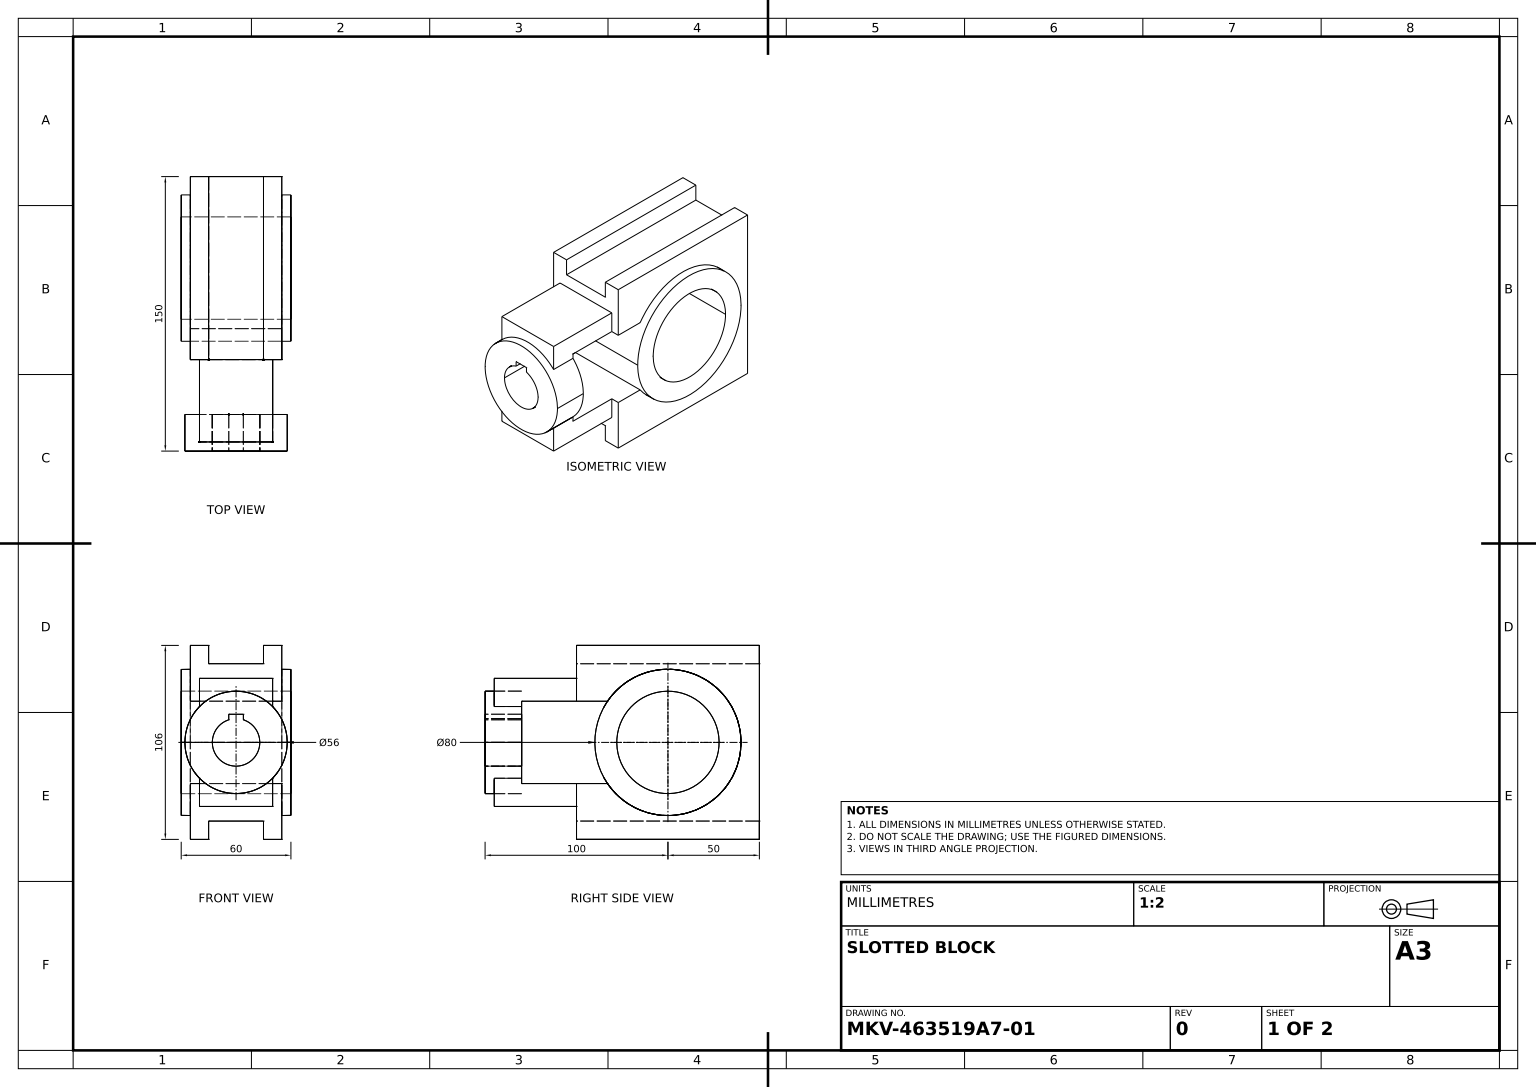
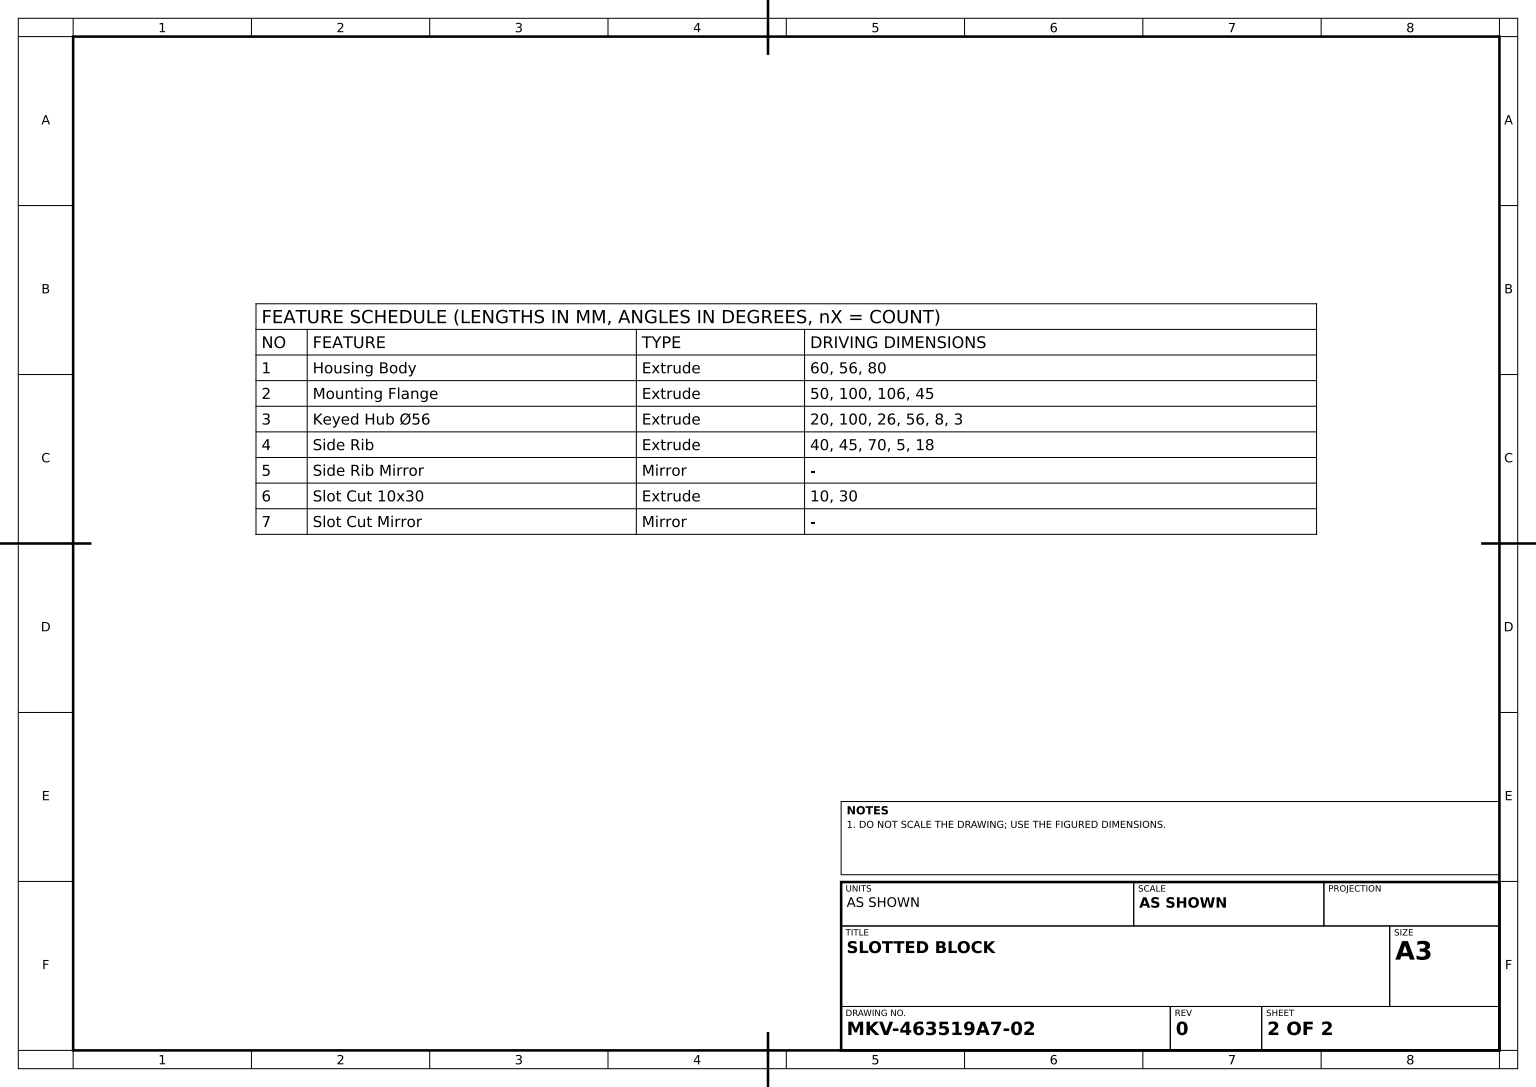
from build123d import *

# Parameters (mm, degrees)
HOUSING_BODY_SKETCH_R   = 40
HOUSING_BODY_SKETCH_R_2 = 28
HOUSING_BODY_DEPTH      = 30
MOUNTING_FLANGE_DEPTH   = 25
KEYED_START             = 100
KEYED_HUB_SKETCH_R      = 28
KEYED_HUB_56_DEPTH      = 20
SIDE_RIB_DEPTH          = 20
SLOT_CUT_SKETCH_W       = 30
SLOT_CUT_SKETCH_H       = 10
SLOT_CUT_10X30_DEPTH    = 118.08543889


with BuildPart() as part:
    # Housing Body Sketch → Housing Body (new, symmetric)
    with BuildSketch(Plane(origin=(0, 0, 0), x_dir=(0, 0, -1), z_dir=(1, 0, 0))):
        Circle(HOUSING_BODY_SKETCH_R)
        Circle(HOUSING_BODY_SKETCH_R_2, mode=Mode.SUBTRACT)
    extrude(amount=HOUSING_BODY_DEPTH, both=True)

    # Mounting Flange Sketch → Mounting Flange (add, symmetric)
    with BuildSketch(Plane(origin=(0, 0, 0), x_dir=(0, 0, -1), z_dir=(1, 0, 0))):
        with BuildLine():
            Line((-33.071891388, -22.5), (-50, -22.5))
            Line((-50, -22.5), (-50, -53))
            Line((-50, -53), (50, -53))
            Line((50, -53), (50, 53))
            Line((50, 53), (-50, 53))
            Line((-50, 53), (-50, 22.5))
            Line((-50, 22.5), (-33.071891388, 22.5))
            ThreePointArc((-33.071891388, 22.5), (11.771243445, 38.228756555), (40, 0))
            ThreePointArc((40, 0), (11.771243445, -38.228756555), (-33.071891388, -22.5))
        make_face()
    extrude(amount=MOUNTING_FLANGE_DEPTH, both=True)



with BuildPart() as body_2:
    # Keyed Hub Sketch → Keyed Hub Ø56 (new body)
    with BuildSketch(Plane.XY.offset(KEYED_START)):
        Circle(KEYED_HUB_SKETCH_R)
        with BuildLine():
            Line((-4, 12.369316877), (-4, 15.369316877))
            Line((-4, 15.369316877), (4, 15.369316877))
            Line((4, 15.369316877), (4, 12.369316877))
            ThreePointArc((4, 12.369316877), (0, -13), (-4, 12.369316877))
        make_face(mode=Mode.SUBTRACT)
    extrude(amount=-KEYED_HUB_56_DEPTH)


with BuildPart() as part_1:
    add(part.part)

    add(body_2.part)  # Side Rib merges body 2
    # Side Rib Sketch → Side Rib (add, symmetric)
    with BuildSketch(Plane(origin=(0, 0, 0), x_dir=(0, 0, -1), z_dir=(1, 0, 0))):
        Polygon((-50, 35), (-95, 35), (-95, 17), (-80, 17), (-80, 22.5), (-50, 22.5), align=None)
    side_rib = extrude(amount=SIDE_RIB_DEPTH, both=True)

    # Side Rib Mirror: Side Rib across plane
    add(side_rib.mirror(Plane.ZX))

    # Slot Cut Sketch → Slot Cut 10x30 (cut, through all)
    with BuildSketch(Plane.XY.offset(50)):
        with Locations((0, 48)):
            Rectangle(SLOT_CUT_SKETCH_W, SLOT_CUT_SKETCH_H)
    slot_cut_10x30 = extrude(amount=-SLOT_CUT_10X30_DEPTH, mode=Mode.SUBTRACT)

    # Slot Cut Mirror: Slot Cut 10x30 across plane
    add(slot_cut_10x30.mirror(Plane.ZX), mode=Mode.SUBTRACT)


solid = part_1.part
